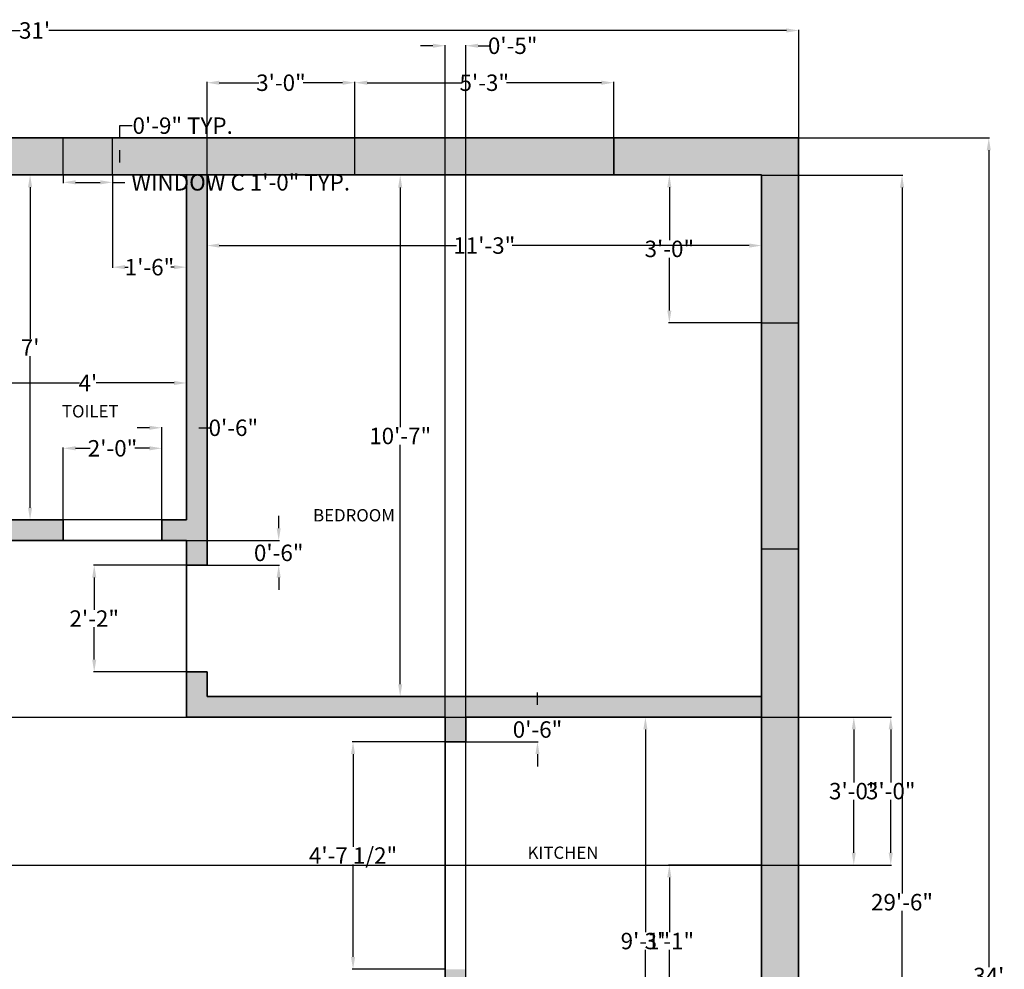
# Model space of a CAD drawing. Units: inches. Extents: x 477 to 929, y 265 to 727.
# Tile 4 of 4: x 690 to 929, y 496 to 727. Entities that reach past the tile are written whole.
import ezdxf

# ---------------------------------------------------------------- set-up
doc = ezdxf.new("R2010")
doc.units = ezdxf.units.IN
doc.header["$MEASUREMENT"] = 0
doc.layers.add('A-ANNO-DIMS', color=215, linetype='Continuous', lineweight=18, true_color=0xa953a0)
doc.layers.add('A-WALL-PATT', color=244, linetype='Continuous', lineweight=13, true_color=0x991b1e)
for name, color, linetype, lineweight in [('A-AREA-IDEN', 3, 'Continuous', 25), ('A-GLAZ', 4, 'Continuous', 25), ('A-GLAZ-PATT', 7, 'Continuous', 13), ('A-WALL', 7, 'Continuous', 35)]:
    doc.layers.add(name, color=color, linetype=linetype, lineweight=lineweight)
doc.styles.get("Standard").update_dxf_attribs({"font": 'arial.ttf'})
doc.dimstyles.get("Standard").update_dxf_attribs({"dimtxt": 4, "dimasz": 3, "dimexe": 0.18, "dimexo": 0.0625, "dimgap": 0.09, "dimtad": 0, "dimtih": 1, "dimtoh": 1, "dimdec": 0, "dimzin": 0, "dimdsep": 46, "dimlunit": 3, "dimtxsty": 'Standard', "dimcen": 0, "dimadec": 0, "dimazin": 0, "dimtfac": 1, "dimtdec": 0, "dimtofl": 0, "dimtmove": 0, "dimatfit": 3, "dimfxl": 1, "dimtolj": 1, "dimtzin": 0, "dimarcsym": 1})

# ---------------------------------------------------------------- blocks, each defined once
blk = doc.blocks.new('*D7')
at = {"layer": 'A-ANNO-DIMS', "color": 0, "lineweight": -2, "transparency": 16777216}
for p, q in [((870.27, 557.21), (841.87, 557.21)), ((842.05, 554.21), (842.05, 504.84)), ((842.05, 451.21), (842.05, 500.57)), ((870.27, 448.21), (841.87, 448.21))]:
    blk.add_line(p, q, dxfattribs=at)
at = {"layer": 'A-ANNO-DIMS', "color": 0, "transparency": 16777216}
for points in [[(841.55, 554.21), (842.55, 554.21), (842.05, 557.21)], [(841.55, 451.21), (842.55, 451.21), (842.05, 448.21)]]:
    blk.add_solid(points, dxfattribs=at)
at = {"layer": 'Defpoints', "color": 0, "transparency": 16777216}
for p in [(870.33, 557.21), (842.05, 448.21), (870.33, 448.21)]:
    blk.add_point(p, dxfattribs=at)
at = {"layer": 'A-ANNO-DIMS', "color": 0, "transparency": 16777216, "insert": (842.05, 502.71), "char_height": 4, "attachment_point": 5}
blk.add_mtext('\\A1;9\'-1"', dxfattribs=at)
blk = doc.blocks.new('*D9')
at = {"layer": 'A-ANNO-DIMS', "color": 0, "lineweight": -2, "transparency": 16777216}
for p, q in [((735.33, 689.14), (735.33, 671.84)), ((870.33, 689.14), (870.33, 671.84)), ((738.33, 672.02), (796.06, 672.02)), ((867.33, 672.02), (809.61, 672.02))]:
    blk.add_line(p, q, dxfattribs=at)
at = {"layer": 'A-ANNO-DIMS', "color": 0, "transparency": 16777216}
for points in [[(738.33, 672.52), (738.33, 671.52), (735.33, 672.02)], [(867.33, 672.52), (867.33, 671.52), (870.33, 672.02)]]:
    blk.add_solid(points, dxfattribs=at)
at = {"layer": 'Defpoints', "color": 0, "transparency": 16777216}
for p in [(735.33, 689.21), (870.33, 689.21), (870.33, 672.02)]:
    blk.add_point(p, dxfattribs=at)
at = {"layer": 'A-ANNO-DIMS', "color": 0, "transparency": 16777216, "insert": (802.83, 672.02), "char_height": 4, "attachment_point": 5}
blk.add_mtext('\\A1;11\'-3"', dxfattribs=at)
blk = doc.blocks.new('*D10')
at = {"layer": 'A-ANNO-DIMS', "color": 0, "lineweight": -2, "transparency": 16777216}
for p, q in [((870.27, 689.14), (782.18, 689.14)), ((782.36, 686.14), (782.36, 627.81)), ((782.36, 565.21), (782.36, 623.54)), ((870.27, 562.21), (782.18, 562.21))]:
    blk.add_line(p, q, dxfattribs=at)
at = {"layer": 'A-ANNO-DIMS', "color": 0, "transparency": 16777216}
for points in [[(781.86, 686.14), (782.86, 686.14), (782.36, 689.14)], [(781.86, 565.21), (782.86, 565.21), (782.36, 562.21)]]:
    blk.add_solid(points, dxfattribs=at)
at = {"layer": 'Defpoints', "color": 0, "transparency": 16777216}
for p in [(870.33, 689.14), (782.36, 562.21), (870.33, 562.21)]:
    blk.add_point(p, dxfattribs=at)
at = {"layer": 'A-ANNO-DIMS', "color": 0, "transparency": 16777216, "insert": (782.36, 625.67), "char_height": 4, "attachment_point": 5}
blk.add_mtext('\\A1;10\'-7"', dxfattribs=at)
blk = doc.blocks.new('*D11')
at = {"layer": 'A-ANNO-DIMS', "color": 0, "lineweight": -2, "transparency": 16777216}
for p, q in [((682.33, 605.27), (682.33, 638.75)), ((685.33, 638.57), (704.32, 638.57)), ((727.33, 638.57), (708.34, 638.57)), ((730.33, 605.27), (730.33, 638.75))]:
    blk.add_line(p, q, dxfattribs=at)
at = {"layer": 'A-ANNO-DIMS', "color": 0, "transparency": 16777216}
for points in [[(685.33, 639.07), (685.33, 638.07), (682.33, 638.57)], [(727.33, 639.07), (727.33, 638.07), (730.33, 638.57)]]:
    blk.add_solid(points, dxfattribs=at)
at = {"layer": 'Defpoints', "color": 0, "transparency": 16777216}
for p in [(730.33, 638.57), (682.33, 605.21), (730.33, 605.21)]:
    blk.add_point(p, dxfattribs=at)
at = {"layer": 'A-ANNO-DIMS', "color": 0, "transparency": 16777216, "insert": (706.33, 638.57), "char_height": 4, "attachment_point": 5}
blk.add_mtext("\\A1;4'", dxfattribs=at)
blk = doc.blocks.new('*D12')
at = {"layer": 'A-ANNO-DIMS', "color": 0, "lineweight": -2, "transparency": 16777216}
for p, q in [((730.27, 689.21), (692.08, 689.21)), ((692.26, 686.21), (692.26, 649.3)), ((692.26, 608.21), (692.26, 645.12)), ((730.27, 605.21), (692.08, 605.21))]:
    blk.add_line(p, q, dxfattribs=at)
at = {"layer": 'A-ANNO-DIMS', "color": 0, "transparency": 16777216}
for points in [[(691.76, 686.21), (692.76, 686.21), (692.26, 689.21)], [(691.76, 608.21), (692.76, 608.21), (692.26, 605.21)]]:
    blk.add_solid(points, dxfattribs=at)
at = {"layer": 'Defpoints', "color": 0, "transparency": 16777216}
for p in [(730.33, 689.21), (692.26, 605.21), (730.33, 605.21)]:
    blk.add_point(p, dxfattribs=at)
at = {"layer": 'A-ANNO-DIMS', "color": 0, "transparency": 16777216, "insert": (692.26, 647.21), "char_height": 4, "attachment_point": 5}
blk.add_mtext("\\A1;7'", dxfattribs=at)
blk = doc.blocks.new('*D17')
at = {"layer": 'A-ANNO-DIMS', "color": 0, "lineweight": -2, "transparency": 16777216}
for p, q in [((879.4, 698.21), (925.82, 698.21)), ((925.64, 695.21), (925.64, 496.34)), ((925.64, 293.21), (925.64, 492.07)), ((879.4, 290.21), (925.82, 290.21))]:
    blk.add_line(p, q, dxfattribs=at)
at = {"layer": 'A-ANNO-DIMS', "color": 0, "transparency": 16777216}
for points in [[(925.14, 695.21), (926.14, 695.21), (925.64, 698.21)], [(925.14, 293.21), (926.14, 293.21), (925.64, 290.21)]]:
    blk.add_solid(points, dxfattribs=at)
at = {"layer": 'Defpoints', "color": 0, "transparency": 16777216}
for p in [(879.33, 698.21), (879.33, 290.21), (925.64, 290.21)]:
    blk.add_point(p, dxfattribs=at)
at = {"layer": 'A-ANNO-DIMS', "color": 0, "transparency": 16777216, "insert": (925.64, 494.21), "char_height": 4, "attachment_point": 5}
blk.add_mtext("\\A1;34'", dxfattribs=at)
blk = doc.blocks.new('*D18')
at = {"layer": 'A-ANNO-DIMS', "color": 0, "lineweight": -2, "transparency": 16777216}
for p, q in [((507.33, 698.27), (507.33, 724.56)), ((510.33, 724.38), (689.88, 724.38)), ((876.4, 724.38), (696.85, 724.38)), ((879.4, 698.27), (879.4, 724.56))]:
    blk.add_line(p, q, dxfattribs=at)
at = {"layer": 'A-ANNO-DIMS', "color": 0, "transparency": 16777216}
for points in [[(510.33, 724.88), (510.33, 723.88), (507.33, 724.38)], [(876.4, 724.88), (876.4, 723.88), (879.4, 724.38)]]:
    blk.add_solid(points, dxfattribs=at)
at = {"layer": 'Defpoints', "color": 0, "transparency": 16777216}
for p in [(879.4, 724.38), (507.33, 698.21), (879.4, 698.21)]:
    blk.add_point(p, dxfattribs=at)
at = {"layer": 'A-ANNO-DIMS', "color": 0, "transparency": 16777216, "insert": (693.36, 724.38), "char_height": 4, "attachment_point": 5}
blk.add_mtext("\\A1;31'", dxfattribs=at)
blk = doc.blocks.new('*D19')
at = {"layer": 'A-ANNO-DIMS', "color": 0, "lineweight": -2, "transparency": 16777216}
for p, q in [((870.4, 689.14), (904.7, 689.14)), ((904.52, 686.14), (904.52, 514.31)), ((904.52, 338.21), (904.52, 510.04)), ((870.33, 335.21), (904.7, 335.21))]:
    blk.add_line(p, q, dxfattribs=at)
at = {"layer": 'A-ANNO-DIMS', "color": 0, "transparency": 16777216}
for points in [[(904.02, 686.14), (905.02, 686.14), (904.52, 689.14)], [(904.02, 338.21), (905.02, 338.21), (904.52, 335.21)]]:
    blk.add_solid(points, dxfattribs=at)
at = {"layer": 'Defpoints', "color": 0, "transparency": 16777216}
for p in [(870.33, 689.14), (870.27, 335.21), (904.52, 335.21)]:
    blk.add_point(p, dxfattribs=at)
at = {"layer": 'A-ANNO-DIMS', "color": 0, "transparency": 16777216, "insert": (904.52, 512.17), "char_height": 4, "attachment_point": 5}
blk.add_mtext('\\A1;29\'-6"', dxfattribs=at)
blk = doc.blocks.new('WIN-JAMBS-55IN')
for p, q in [((0, 55), (9, 55)), ((0, 0), (9, 0))]:
    blk.add_line(p, q)
blk = doc.blocks.new('WIN-JAMBS-12IN')
for p, q in [((0, 0), (0, 9)), ((12, 0), (12, 9))]:
    blk.add_line(p, q)
blk = doc.blocks.new('*D27')
at = {"layer": 'A-ANNO-DIMS', "color": 0, "lineweight": -2, "transparency": 16777216}
for p, q in [((700.33, 689.14), (700.33, 687.23)), ((712.33, 689.14), (712.33, 687.23)), ((703.33, 687.41), (709.33, 687.41)), ((712.33, 687.41), (715.33, 687.41))]:
    blk.add_line(p, q, dxfattribs=at)
at = {"layer": 'A-ANNO-DIMS', "color": 0, "transparency": 16777216}
for points in [[(703.33, 687.91), (703.33, 686.91), (700.33, 687.41)], [(709.33, 687.91), (709.33, 686.91), (712.33, 687.41)]]:
    blk.add_solid(points, dxfattribs=at)
at = {"layer": 'Defpoints', "color": 0, "transparency": 16777216}
for p in [(700.33, 689.21), (712.33, 689.21), (712.33, 687.41)]:
    blk.add_point(p, dxfattribs=at)
at = {"layer": 'A-ANNO-DIMS', "color": 0, "transparency": 16777216, "insert": (743.53, 687.41), "char_height": 4, "attachment_point": 5}
blk.add_mtext('\\A1;WINDOW C 1\'-0" TYP.', dxfattribs=at)
blk = doc.blocks.new('*D28')
at = {"layer": 'A-ANNO-DIMS', "color": 0, "lineweight": -2, "transparency": 16777216}
for p, q in [((714.13, 698.21), (714.13, 701.21)), ((714.13, 701.21), (717.13, 701.21)), ((712.4, 698.21), (714.31, 698.21)), ((714.13, 692.21), (714.13, 695.21)), ((712.4, 689.21), (714.31, 689.21))]:
    blk.add_line(p, q, dxfattribs=at)
at = {"layer": 'A-ANNO-DIMS', "color": 0, "transparency": 16777216}
for points in [[(713.63, 695.21), (714.63, 695.21), (714.13, 698.21)], [(713.63, 692.21), (714.63, 692.21), (714.13, 689.21)]]:
    blk.add_solid(points, dxfattribs=at)
at = {"layer": 'Defpoints', "color": 0, "transparency": 16777216}
for p in [(712.33, 698.21), (714.13, 698.21), (712.33, 689.21)]:
    blk.add_point(p, dxfattribs=at)
at = {"layer": 'A-ANNO-DIMS', "color": 0, "transparency": 16777216, "insert": (729.41, 701.21), "char_height": 4, "attachment_point": 5}
blk.add_mtext('\\A1;0\'-9" TYP.', dxfattribs=at)
blk = doc.blocks.new('*D30')
at = {"layer": 'A-ANNO-DIMS', "color": 0, "lineweight": -2, "transparency": 16777216}
for p, q in [((588.43, 557.21), (901.96, 557.21)), ((901.78, 554.21), (901.78, 541.34)), ((901.78, 524.21), (901.78, 537.07)), ((588.43, 521.21), (901.96, 521.21))]:
    blk.add_line(p, q, dxfattribs=at)
at = {"layer": 'A-ANNO-DIMS', "color": 0, "transparency": 16777216}
for points in [[(901.28, 554.21), (902.28, 554.21), (901.78, 557.21)], [(901.28, 524.21), (902.28, 524.21), (901.78, 521.21)]]:
    blk.add_solid(points, dxfattribs=at)
at = {"layer": 'Defpoints', "color": 0, "transparency": 16777216}
for p in [(588.37, 557.21), (901.78, 557.21), (588.37, 521.21)]:
    blk.add_point(p, dxfattribs=at)
at = {"layer": 'A-ANNO-DIMS', "color": 0, "transparency": 16777216, "insert": (901.78, 539.21), "char_height": 4, "attachment_point": 5}
blk.add_mtext('\\A1;3\'-0"', dxfattribs=at)
blk = doc.blocks.new('*D39')
at = {"layer": 'A-ANNO-DIMS', "color": 0, "lineweight": -2, "transparency": 16777216}
for p, q in [((790.33, 720.66), (787.33, 720.66)), ((793.33, 448.27), (793.33, 720.84)), ((798.33, 448.27), (798.33, 720.84)), ((801.33, 720.66), (804.33, 720.66))]:
    blk.add_line(p, q, dxfattribs=at)
at = {"layer": 'A-ANNO-DIMS', "color": 0, "transparency": 16777216}
for points in [[(790.33, 721.16), (790.33, 720.16), (793.33, 720.66)], [(801.33, 721.16), (801.33, 720.16), (798.33, 720.66)]]:
    blk.add_solid(points, dxfattribs=at)
at = {"layer": 'Defpoints', "color": 0, "transparency": 16777216}
for p in [(798.33, 720.66), (793.33, 448.21), (798.33, 448.21)]:
    blk.add_point(p, dxfattribs=at)
at = {"layer": 'A-ANNO-DIMS', "color": 0, "transparency": 16777216, "insert": (809.74, 720.66), "char_height": 4, "attachment_point": 5}
blk.add_mtext('\\A1;0\'-5"', dxfattribs=at)
blk = doc.blocks.new('*D42')
at = {"layer": 'A-ANNO-DIMS', "color": 0, "lineweight": -2, "transparency": 16777216}
for p, q in [((712.33, 689.14), (712.33, 666.58)), ((730.33, 689.14), (730.33, 666.58)), ((715.33, 666.76), (716.12, 666.76)), ((727.33, 666.76), (726.55, 666.76))]:
    blk.add_line(p, q, dxfattribs=at)
at = {"layer": 'A-ANNO-DIMS', "color": 0, "transparency": 16777216}
for points in [[(715.33, 667.26), (715.33, 666.26), (712.33, 666.76)], [(727.33, 667.26), (727.33, 666.26), (730.33, 666.76)]]:
    blk.add_solid(points, dxfattribs=at)
at = {"layer": 'Defpoints', "color": 0, "transparency": 16777216}
for p in [(712.33, 689.21), (730.33, 689.21), (712.33, 666.76)]:
    blk.add_point(p, dxfattribs=at)
at = {"layer": 'A-ANNO-DIMS', "color": 0, "transparency": 16777216, "insert": (721.33, 666.76), "char_height": 4, "attachment_point": 5}
blk.add_mtext('\\A1;1\'-6"', dxfattribs=at)
blk = doc.blocks.new('*D43')
at = {"layer": 'A-ANNO-DIMS', "color": 0, "lineweight": -2, "transparency": 16777216}
for p, q in [((735.33, 689.27), (735.33, 711.84)), ((738.33, 711.66), (747.93, 711.66)), ((768.33, 711.66), (758.74, 711.66)), ((771.33, 689.27), (771.33, 711.84))]:
    blk.add_line(p, q, dxfattribs=at)
at = {"layer": 'A-ANNO-DIMS', "color": 0, "transparency": 16777216}
for points in [[(738.33, 712.16), (738.33, 711.16), (735.33, 711.66)], [(768.33, 712.16), (768.33, 711.16), (771.33, 711.66)]]:
    blk.add_solid(points, dxfattribs=at)
at = {"layer": 'Defpoints', "color": 0, "transparency": 16777216}
for p in [(771.33, 711.66), (735.33, 689.21), (771.33, 689.21)]:
    blk.add_point(p, dxfattribs=at)
at = {"layer": 'A-ANNO-DIMS', "color": 0, "transparency": 16777216, "insert": (753.33, 711.66), "char_height": 4, "attachment_point": 5}
blk.add_mtext('\\A1;3\'-0"', dxfattribs=at)
blk = doc.blocks.new('*D44')
at = {"layer": 'A-ANNO-DIMS', "color": 0, "lineweight": -2, "transparency": 16777216}
for p, q in [((771.33, 689.27), (771.33, 711.84)), ((774.33, 711.66), (797.43, 711.66)), ((831.33, 711.66), (808.24, 711.66)), ((834.33, 689.27), (834.33, 711.84))]:
    blk.add_line(p, q, dxfattribs=at)
at = {"layer": 'A-ANNO-DIMS', "color": 0, "transparency": 16777216}
for points in [[(774.33, 712.16), (774.33, 711.16), (771.33, 711.66)], [(831.33, 712.16), (831.33, 711.16), (834.33, 711.66)]]:
    blk.add_solid(points, dxfattribs=at)
at = {"layer": 'Defpoints', "color": 0, "transparency": 16777216}
for p in [(834.33, 711.66), (771.33, 689.21), (834.33, 689.21)]:
    blk.add_point(p, dxfattribs=at)
at = {"layer": 'A-ANNO-DIMS', "color": 0, "transparency": 16777216, "insert": (802.83, 711.66), "char_height": 4, "attachment_point": 5}
blk.add_mtext('\\A1;5\'-3"', dxfattribs=at)
blk = doc.blocks.new('*D50')
at = {"layer": 'A-ANNO-DIMS', "color": 0, "lineweight": -2, "transparency": 16777216}
for p, q in [((870.27, 689.21), (847.7, 689.21)), ((847.88, 686.21), (847.88, 673.34)), ((847.88, 656.21), (847.88, 669.07)), ((870.27, 653.21), (847.7, 653.21))]:
    blk.add_line(p, q, dxfattribs=at)
at = {"layer": 'A-ANNO-DIMS', "color": 0, "transparency": 16777216}
for points in [[(847.38, 686.21), (848.38, 686.21), (847.88, 689.21)], [(847.38, 656.21), (848.38, 656.21), (847.88, 653.21)]]:
    blk.add_solid(points, dxfattribs=at)
at = {"layer": 'Defpoints', "color": 0, "transparency": 16777216}
for p in [(847.88, 689.21), (870.33, 689.21), (870.33, 653.21)]:
    blk.add_point(p, dxfattribs=at)
at = {"layer": 'A-ANNO-DIMS', "color": 0, "transparency": 16777216, "insert": (847.88, 671.21), "char_height": 4, "attachment_point": 5}
blk.add_mtext('\\A1;3\'-0"', dxfattribs=at)
blk = doc.blocks.new('*D51')
at = {"layer": 'A-ANNO-DIMS', "color": 0, "lineweight": -2, "transparency": 16777216}
for p, q in [((870.4, 557.21), (892.96, 557.21)), ((892.78, 554.21), (892.78, 541.34)), ((892.78, 524.21), (892.78, 537.07)), ((870.4, 521.21), (892.96, 521.21))]:
    blk.add_line(p, q, dxfattribs=at)
at = {"layer": 'A-ANNO-DIMS', "color": 0, "transparency": 16777216}
for points in [[(892.28, 554.21), (893.28, 554.21), (892.78, 557.21)], [(892.28, 524.21), (893.28, 524.21), (892.78, 521.21)]]:
    blk.add_solid(points, dxfattribs=at)
at = {"layer": 'Defpoints', "color": 0, "transparency": 16777216}
for p in [(870.33, 557.21), (870.33, 521.21), (892.78, 521.21)]:
    blk.add_point(p, dxfattribs=at)
at = {"layer": 'A-ANNO-DIMS', "color": 0, "transparency": 16777216, "insert": (892.78, 539.21), "char_height": 4, "attachment_point": 5}
blk.add_mtext('\\A1;3\'-0"', dxfattribs=at)
blk = doc.blocks.new('*D52')
at = {"layer": 'A-ANNO-DIMS', "color": 0, "lineweight": -2, "transparency": 16777216}
for p, q in [((870.27, 521.21), (847.7, 521.21)), ((847.88, 518.21), (847.88, 504.84)), ((847.88, 487.21), (847.88, 500.57)), ((870.27, 484.21), (847.7, 484.21))]:
    blk.add_line(p, q, dxfattribs=at)
at = {"layer": 'A-ANNO-DIMS', "color": 0, "transparency": 16777216}
for points in [[(847.38, 518.21), (848.38, 518.21), (847.88, 521.21)], [(847.38, 487.21), (848.38, 487.21), (847.88, 484.21)]]:
    blk.add_solid(points, dxfattribs=at)
at = {"layer": 'Defpoints', "color": 0, "transparency": 16777216}
for p in [(847.88, 521.21), (870.33, 521.21), (870.33, 484.21)]:
    blk.add_point(p, dxfattribs=at)
at = {"layer": 'A-ANNO-DIMS', "color": 0, "transparency": 16777216, "insert": (847.88, 502.71), "char_height": 4, "attachment_point": 5}
blk.add_mtext('\\A1;3\'-1"', dxfattribs=at)
blk = doc.blocks.new('*D59')
at = {"layer": 'A-ANNO-DIMS', "color": 0, "lineweight": -2, "transparency": 16777216}
for p, q in [((793.27, 551.21), (770.7, 551.21)), ((770.88, 548.21), (770.88, 525.68)), ((770.88, 498.83), (770.88, 521.36)), ((793.27, 495.83), (770.7, 495.83))]:
    blk.add_line(p, q, dxfattribs=at)
at = {"layer": 'A-ANNO-DIMS', "color": 0, "transparency": 16777216}
for points in [[(770.38, 548.21), (771.38, 548.21), (770.88, 551.21)], [(770.38, 498.83), (771.38, 498.83), (770.88, 495.83)]]:
    blk.add_solid(points, dxfattribs=at)
at = {"layer": 'Defpoints', "color": 0, "transparency": 16777216}
for p in [(770.88, 551.21), (793.33, 551.21), (793.33, 495.83)]:
    blk.add_point(p, dxfattribs=at)
at = {"layer": 'A-ANNO-DIMS', "color": 0, "transparency": 16777216, "insert": (770.88, 523.52), "char_height": 4, "attachment_point": 5}
blk.add_mtext('\\A1;4\'-7 1/2"', dxfattribs=at)
blk = doc.blocks.new('*D60')
at = {"layer": 'A-ANNO-DIMS', "color": 0, "lineweight": -2, "transparency": 16777216}
for p, q in [((730.27, 594.21), (707.7, 594.21)), ((707.88, 591.21), (707.88, 583.3)), ((707.88, 571.21), (707.88, 579.11)), ((730.27, 568.21), (707.7, 568.21))]:
    blk.add_line(p, q, dxfattribs=at)
at = {"layer": 'A-ANNO-DIMS', "color": 0, "transparency": 16777216}
for points in [[(707.38, 591.21), (708.38, 591.21), (707.88, 594.21)], [(707.38, 571.21), (708.38, 571.21), (707.88, 568.21)]]:
    blk.add_solid(points, dxfattribs=at)
at = {"layer": 'Defpoints', "color": 0, "transparency": 16777216}
for p in [(707.88, 594.21), (730.33, 594.21), (730.33, 568.21)]:
    blk.add_point(p, dxfattribs=at)
at = {"layer": 'A-ANNO-DIMS', "color": 0, "transparency": 16777216, "insert": (707.88, 581.21), "char_height": 4, "attachment_point": 5}
blk.add_mtext('\\A1;2\'-2"', dxfattribs=at)
blk = doc.blocks.new('*D62')
at = {"layer": 'A-ANNO-DIMS', "color": 0, "lineweight": -2, "transparency": 16777216}
for p, q in [((700.33, 600.27), (700.33, 622.84)), ((703.33, 622.66), (706.89, 622.66)), ((721.33, 622.66), (717.77, 622.66)), ((724.33, 600.27), (724.33, 622.84))]:
    blk.add_line(p, q, dxfattribs=at)
at = {"layer": 'A-ANNO-DIMS', "color": 0, "transparency": 16777216}
for points in [[(703.33, 623.16), (703.33, 622.16), (700.33, 622.66)], [(721.33, 623.16), (721.33, 622.16), (724.33, 622.66)]]:
    blk.add_solid(points, dxfattribs=at)
at = {"layer": 'Defpoints', "color": 0, "transparency": 16777216}
for p in [(724.33, 622.66), (700.33, 600.21), (724.33, 600.21)]:
    blk.add_point(p, dxfattribs=at)
at = {"layer": 'A-ANNO-DIMS', "color": 0, "transparency": 16777216, "insert": (712.33, 622.66), "char_height": 4, "attachment_point": 5}
blk.add_mtext('\\A1;2\'-0"', dxfattribs=at)
blk = doc.blocks.new('*D66')
at = {"layer": 'A-ANNO-DIMS', "color": 0, "lineweight": -2, "transparency": 16777216}
for p, q in [((752.783739, 603.205163), (752.783739, 606.205163)), ((730.396239, 600.205163), (752.963739, 600.205163)), ((730.396239, 594.205163), (752.963739, 594.205163)), ((752.783739, 591.205163), (752.783739, 588.205163))]:
    blk.add_line(p, q, dxfattribs=at)
at = {"layer": 'A-ANNO-DIMS', "color": 0, "transparency": 16777216}
for points in [[(752.283739, 603.205163), (753.283739, 603.205163), (752.783739, 600.205163)], [(752.283739, 591.205163), (753.283739, 591.205163), (752.783739, 594.205163)]]:
    blk.add_solid(points, dxfattribs=at)
at = {"layer": 'Defpoints', "color": 0, "transparency": 16777216}
for p in [(730.333739, 600.205163), (730.333739, 594.205163), (752.783739, 594.205163)]:
    blk.add_point(p, dxfattribs=at)
at = {"layer": 'A-ANNO-DIMS', "color": 0, "transparency": 16777216, "insert": (752.783739, 597.205163), "char_height": 4, "attachment_point": 5}
blk.add_mtext('\\A1;0\'-6"', dxfattribs=at)
blk = doc.blocks.new('*D69')
at = {"layer": 'A-ANNO-DIMS', "color": 0, "lineweight": -2, "transparency": 16777216}
for p, q in [((721.33, 627.66), (718.33, 627.66)), ((724.33, 605.27), (724.33, 627.84)), ((730.33, 605.27), (730.33, 627.84)), ((733.33, 627.66), (736.33, 627.66))]:
    blk.add_line(p, q, dxfattribs=at)
at = {"layer": 'A-ANNO-DIMS', "color": 0, "transparency": 16777216}
for points in [[(721.33, 628.16), (721.33, 627.16), (724.33, 627.66)], [(733.33, 628.16), (733.33, 627.16), (730.33, 627.66)]]:
    blk.add_solid(points, dxfattribs=at)
at = {"layer": 'Defpoints', "color": 0, "transparency": 16777216}
for p in [(730.33, 627.66), (724.33, 605.21), (730.33, 605.21)]:
    blk.add_point(p, dxfattribs=at)
at = {"layer": 'A-ANNO-DIMS', "color": 0, "transparency": 16777216, "insert": (741.74, 627.66), "char_height": 4, "attachment_point": 5}
blk.add_mtext('\\A1;0\'-6"', dxfattribs=at)
blk = doc.blocks.new('*D70')
at = {"layer": 'A-ANNO-DIMS', "color": 0, "lineweight": -2, "transparency": 16777216}
for p, q in [((815.783739, 560.205163), (815.783739, 563.205163)), ((793.396239, 557.205163), (815.963739, 557.205163)), ((793.396239, 551.205163), (815.963739, 551.205163)), ((815.783739, 548.205163), (815.783739, 545.205163))]:
    blk.add_line(p, q, dxfattribs=at)
at = {"layer": 'A-ANNO-DIMS', "color": 0, "transparency": 16777216}
for points in [[(815.283739, 560.205163), (816.283739, 560.205163), (815.783739, 557.205163)], [(815.283739, 548.205163), (816.283739, 548.205163), (815.783739, 551.205163)]]:
    blk.add_solid(points, dxfattribs=at)
at = {"layer": 'Defpoints', "color": 0, "transparency": 16777216}
for p in [(793.333739, 557.205163), (793.333739, 551.205163), (815.783739, 551.205163)]:
    blk.add_point(p, dxfattribs=at)
at = {"layer": 'A-ANNO-DIMS', "color": 0, "transparency": 16777216, "insert": (815.783739, 554.205163), "char_height": 4, "attachment_point": 5}
blk.add_mtext('\\A1;0\'-6"', dxfattribs=at)

msp = doc.modelspace()

# ---------------------------------------------------------------- hatches: boundary and pattern name
at = {"layer": 'A-GLAZ-PATT'}
h = msp.add_hatch(color=256, dxfattribs=at)
h.dxf.hatch_style = 1
h.paths.add_polyline_path([(588.33, 698.21), (552.33, 698.21), (552.33, 689.21), (588.33, 689.21)])
h.paths.add_polyline_path([(659.33, 698.21), (647.33, 698.21), (647.33, 689.21), (659.33, 689.21)])
h.paths.add_polyline_path([(712.33, 698.21), (700.33, 698.21), (700.33, 689.21), (712.33, 689.21)])
h.paths.add_polyline_path([(834.33, 698.21), (771.33, 698.21), (771.33, 689.21), (834.33, 689.21)])
h.paths.add_polyline_path([(879.33, 653.21), (870.33, 653.21), (870.33, 598.21), (879.33, 598.21)])
h.paths.add_polyline_path([(879.33, 521.21), (870.33, 521.21), (870.33, 484.21), (879.33, 484.21)])
h.paths.add_polyline_path([(879.33, 407.21), (870.33, 407.21), (870.33, 371.21), (879.33, 371.21)])
h.paths.add_polyline_path([(834.33, 335.21), (766.33, 335.21), (766.33, 326.21), (834.33, 326.21)])
h.paths.add_polyline_path([(588.33, 335.21), (552.33, 335.21), (552.33, 326.21), (588.33, 326.21)])
h.paths.add_polyline_path([(516.33, 430.21), (507.33, 430.21), (507.33, 371.21), (516.33, 371.21)])
h.paths.add_polyline_path([(516.33, 539.21), (507.33, 539.21), (507.33, 466.21), (516.33, 466.21)])
h.paths.add_polyline_path([(516.33, 653.21), (507.33, 653.21), (507.33, 598.21), (516.33, 598.21)])
at = {"layer": 'A-WALL-PATT'}
h = msp.add_hatch(color=256, dxfattribs=at)
h.dxf.hatch_style = 1
h.paths.add_polyline_path([(516.33, 598.21), (507.33, 598.21), (507.33, 539.21), (516.33, 539.21), (516.33, 557.21), (570.33, 557.21), (570.33, 562.21), (516.33, 562.21)])
h.paths.add_polyline_path([(552.33, 698.21), (507.33, 698.21), (507.33, 653.21), (516.33, 653.21), (516.33, 689.21), (552.33, 689.21)])
h.paths.add_polyline_path([(647.33, 698.21), (588.33, 698.21), (588.33, 689.21), (647.33, 689.21)])
h.paths.add_polyline_path([(700.33, 698.21), (659.33, 698.21), (659.33, 689.21), (700.33, 689.21)])
h.paths.add_polyline_path([(771.33, 698.21), (712.33, 698.21), (712.33, 689.21), (771.33, 689.21)])
h.paths.add_polyline_path([(879.33, 698.21), (834.33, 698.21), (834.33, 689.21), (870.33, 689.21), (870.33, 653.21), (879.33, 653.21)])
h.paths.add_polyline_path([(879.33, 598.21), (870.33, 598.21), (870.33, 562.21), (735.33, 562.21), (735.33, 568.21), (730.33, 568.21), (730.33, 557.21), (793.33, 557.21), (793.33, 551.21), (798.33, 551.21), (798.33, 557.21), (870.33, 557.21), (870.33, 521.21), (879.33, 521.21)])
h.paths.add_polyline_path([(879.33, 484.21), (870.33, 484.21), (870.33, 448.21), (798.33, 448.21), (798.33, 495.83), (793.33, 495.83), (793.33, 448.21), (788.33, 448.21), (788.33, 443.21), (870.33, 443.21), (870.33, 407.21), (879.33, 407.21)])
h.paths.add_polyline_path([(735.33, 443.21), (740.33, 443.21), (740.33, 448.21), (730.33, 448.21), (730.33, 400.21), (682.33, 400.21), (682.33, 395.21), (730.33, 395.21), (730.33, 326.21), (766.33, 326.21), (766.33, 335.21), (735.33, 335.21)])
h.paths.add_polyline_path([(879.33, 371.21), (870.33, 371.21), (870.33, 335.21), (834.33, 335.21), (834.33, 326.21), (879.33, 326.21)])
h.paths.add_polyline_path([(516.33, 466.21), (507.33, 466.21), (507.33, 430.21), (516.33, 430.21), (516.33, 443.21), (624.33, 443.21), (624.33, 437.21), (629.33, 437.21), (629.33, 448.21), (516.33, 448.21)])
h.paths.add_polyline_path([(629.33, 600.21), (700.33, 600.21), (700.33, 605.21), (682.33, 605.21), (682.33, 689.21), (677.33, 689.21), (677.33, 605.21), (629.33, 605.21), (629.33, 611.21), (624.33, 611.21), (624.33, 562.21), (618.33, 562.21), (618.33, 557.21), (629.33, 557.21)])
h.paths.add_polyline_path([(629.33, 689.21), (624.33, 689.21), (624.33, 653.21), (629.33, 653.21)], flags=17)
h = msp.add_hatch(color=256, dxfattribs=at)
h.dxf.hatch_style = 1
h.paths.add_polyline_path([(735.33, 689.21), (730.33, 689.21), (730.33, 605.21), (724.33, 605.21), (724.33, 600.21), (730.33, 600.21), (730.33, 594.21), (735.33, 594.21)])

# ---------------------------------------------------------------- linework, layer by layer
at = {"layer": 'A-GLAZ'}
for p, q in [((771.33, 689.21), (771.33, 698.21)), ((834.33, 698.21), (834.33, 689.21)), ((870.33, 521.21), (879.33, 521.21))]:
    msp.add_line(p, q, dxfattribs=at)
at = {"layer": 'A-WALL'}
for p, q in [((507.33, 698.21), (879.33, 698.21)), ((879.33, 698.21), (507.33, 698.21)), ((879.33, 698.21), (879.33, 326.21)), ((879.33, 698.21), (879.33, 326.21)), ((516.33, 689.21), (870.33, 689.21)), ((516.33, 689.21), (870.33, 689.21)), ((730.33, 605.21), (730.33, 689.21)), ((735.33, 594.21), (735.33, 689.21)), ((870.33, 689.21), (870.33, 448.21)), ((682.33, 605.21), (700.33, 605.21)), ((700.33, 600.21), (700.33, 605.21)), ((724.33, 600.21), (724.33, 605.21)), ((724.33, 605.21), (730.33, 605.21)), ((629.33, 600.21), (730.33, 600.21)), ((730.33, 557.21), (730.33, 600.21)), ((730.33, 594.21), (735.33, 594.21)), ((730.33, 568.21), (735.33, 568.21)), ((735.33, 562.21), (735.33, 568.21)), ((735.33, 562.21), (870.33, 562.21)), ((782.18, 562.21), (870.33, 562.21)), ((730.33, 557.21), (793.33, 557.21)), ((793.33, 557.21), (793.33, 448.21)), ((798.33, 557.21), (798.33, 551.21)), ((798.33, 557.21), (870.33, 557.21)), ((841.87, 557.21), (870.27, 557.21)), ((870.33, 557.21), (870.33, 448.21)), ((793.33, 551.21), (798.33, 551.21))]:
    msp.add_line(p, q, dxfattribs=at)

# ---------------------------------------------------------------- block references
at = {"layer": 'A-GLAZ'}
for name, p in [('WIN-JAMBS-12IN', (700.33, 689.21)), ('WIN-JAMBS-55IN', (870.33, 598.21))]:
    msp.add_blockref(name, p, dxfattribs=at)

# ---------------------------------------------------------------- texts
at = {"layer": 'A-AREA-IDEN'}
for s, p in [('TOILET', (700.02, 630.17)), ('KITCHEN', (813.37, 522.72))]:
    msp.add_text(s, height=3, dxfattribs=at).set_placement(p)
at = {"layer": 'A-AREA-IDEN', "insert": (761.16, 607.86), "char_height": 3, "attachment_point": 1}
msp.add_mtext_dynamic_manual_height_columns('BEDROOM', width=102.2555, gutter_width=1, heights=[0], dxfattribs=at)

# ---------------------------------------------------------------- dimensions: what is measured, and where the dimension line sits
at = {"layer": 'A-ANNO-DIMS'}
for base, p1, p2, override, picture, middle in [((879.4, 724.38), (507.33, 698.21), (879.4, 698.21), {"dimclrd": 0, "dimclre": 0, "dimclrt": 0}, '*D18', (693.36, 724.38)), ((798.33, 720.66), (793.33, 448.21), (798.33, 448.21), {"dimdec": 1, "dimlfac": 1, "dimrnd": 0, "dimzin": 1, "dimdsep": 46, "dimlunit": 4, "dimfrac": 2}, '*D39', (809.74, 720.66)), ((834.33, 711.66), (771.33, 689.21), (834.33, 689.21), {"dimdec": 1, "dimlfac": 1, "dimrnd": 0, "dimzin": 1, "dimdsep": 46, "dimlunit": 4, "dimfrac": 2}, '*D44', (802.83, 711.66)), ((870.33, 672.02), (735.33, 689.21), (870.33, 689.21), {"dimclrd": 0, "dimclre": 0, "dimclrt": 0}, '*D9', (802.83, 672.02)), ((730.33, 638.57), (682.33, 605.21), (730.33, 605.21), {"dimclrd": 0, "dimclre": 0, "dimclrt": 0}, '*D11', (706.33, 638.57)), ((730.33, 627.66), (724.33, 605.21), (730.33, 605.21), {"dimdec": 1, "dimlfac": 1, "dimrnd": 0, "dimzin": 1, "dimdsep": 46, "dimlunit": 4, "dimfrac": 2}, '*D69', (741.74, 627.66)), ((724.33, 622.66), (700.33, 600.21), (724.33, 600.21), {"dimdec": 1, "dimlfac": 1, "dimrnd": 0, "dimzin": 1, "dimdsep": 46, "dimlunit": 4, "dimfrac": 2}, '*D62', (712.33, 622.66))]:
    dim = msp.add_linear_dim(base=base, p1=p1, p2=p2, dimstyle='Standard', override=override, dxfattribs=at)
    dim.commit()
    dim.dimension.update_dxf_attribs({"geometry": picture, "text_midpoint": middle})
for base, p1, p2, angle, override, picture, middle in [((771.33, 711.66), (735.33, 689.21), (771.33, 689.21), 0, {"dimdec": 1, "dimlfac": 1, "dimrnd": 0, "dimzin": 1, "dimdsep": 46, "dimlunit": 4, "dimfrac": 2}, '*D43', (753.33, 711.66)), ((925.64, 290.21), (879.33, 698.21), (879.33, 290.21), 90, {"dimclrd": 0, "dimclre": 0, "dimclrt": 0}, '*D17', (925.64, 494.21)), ((692.26, 605.21), (730.33, 689.21), (730.33, 605.21), 90, {"dimclrd": 0, "dimclre": 0, "dimclrt": 0}, '*D12', (692.26, 647.21)), ((712.33, 666.76), (730.33, 689.21), (712.33, 689.21), 180, {"dimdec": 1, "dimlfac": 1, "dimrnd": 0, "dimzin": 1, "dimdsep": 46, "dimlunit": 4, "dimfrac": 2}, '*D42', (721.33, 666.76)), ((782.36, 562.21), (870.33, 689.14), (870.33, 562.21), 90, {"dimclrd": 0, "dimclre": 0, "dimclrt": 0}, '*D10', (782.36, 625.67)), ((847.88, 689.21), (870.33, 653.21), (870.33, 689.21), 90, {"dimdec": 1, "dimlfac": 1, "dimrnd": 0, "dimzin": 1, "dimdsep": 46, "dimlunit": 4, "dimfrac": 2}, '*D50', (847.88, 671.21)), ((904.52, 335.21), (870.33, 689.14), (870.27, 335.21), 90, {"dimclrd": 0, "dimclre": 0, "dimclrt": 0}, '*D19', (904.52, 512.17)), ((752.78, 594.21), (730.33, 600.21), (730.33, 594.21), 270, {"dimdec": 1, "dimlfac": 1, "dimrnd": 0, "dimzin": 1, "dimdsep": 46, "dimlunit": 4, "dimfrac": 2}, '*D66', (752.78, 597.21)), ((707.88, 594.21), (730.33, 568.21), (730.33, 594.21), 90, {"dimdec": 1, "dimlfac": 1, "dimrnd": 0, "dimzin": 1, "dimdsep": 46, "dimlunit": 4, "dimfrac": 2}, '*D60', (707.88, 581.21)), ((815.78, 551.21), (793.33, 557.21), (793.33, 551.21), 270, {"dimdec": 1, "dimlfac": 1, "dimrnd": 0, "dimzin": 1, "dimdsep": 46, "dimlunit": 4, "dimfrac": 2}, '*D70', (815.78, 554.21)), ((901.78, 557.21), (588.37, 521.21), (588.37, 557.21), 90, {"dimdec": 1, "dimlfac": 1, "dimrnd": 0, "dimzin": 1, "dimdsep": 46, "dimlunit": 4, "dimfrac": 2}, '*D30', (901.78, 539.21)), ((842.05, 448.21), (870.33, 557.21), (870.33, 448.21), 90, {"dimclrd": 0, "dimclre": 0, "dimclrt": 0}, '*D7', (842.05, 502.71)), ((892.78, 521.21), (870.33, 557.21), (870.33, 521.21), 270, {"dimdec": 1, "dimlfac": 1, "dimrnd": 0, "dimzin": 1, "dimdsep": 46, "dimlunit": 4, "dimfrac": 2}, '*D51', (892.78, 539.21)), ((770.88, 551.21), (793.33, 495.83), (793.33, 551.21), 90, {"dimdec": 1, "dimlfac": 1, "dimrnd": 0, "dimzin": 1, "dimdsep": 46, "dimlunit": 4, "dimfrac": 2}, '*D59', (770.88, 523.52)), ((847.88, 521.21), (870.33, 484.21), (870.33, 521.21), 90, {"dimdec": 1, "dimlfac": 1, "dimrnd": 0, "dimzin": 1, "dimdsep": 46, "dimlunit": 4, "dimfrac": 2}, '*D52', (847.88, 502.71))]:
    dim = msp.add_linear_dim(base=base, p1=p1, p2=p2, angle=angle, dimstyle='Standard', override=override, dxfattribs=at)
    dim.commit()
    dim.dimension.update_dxf_attribs({"geometry": picture, "text_midpoint": middle})
dim = msp.add_linear_dim(base=(714.13, 698.21), p1=(712.33, 689.21), p2=(712.33, 698.21), angle=90, text='<> TYP.', dimstyle='Standard', override={"dimdec": 1, "dimlfac": 1, "dimrnd": 0, "dimzin": 1, "dimdsep": 46, "dimlunit": 4, "dimfrac": 2}, dxfattribs=at)
dim.commit()
dim.dimension.update_dxf_attribs({"geometry": '*D28', "text_midpoint": (729.41, 701.21)})
dim = msp.add_linear_dim(base=(712.33, 687.41), p1=(700.33, 689.21), p2=(712.33, 689.21), text='WINDOW C <> TYP.', dimstyle='Standard', override={"dimdec": 1, "dimlfac": 1, "dimrnd": 0, "dimzin": 1, "dimdsep": 46, "dimlunit": 4, "dimfrac": 2}, dxfattribs=at)
dim.commit()
dim.dimension.update_dxf_attribs({"geometry": '*D27', "text_midpoint": (743.53, 687.41)})

doc.saveas('drawing.dxf')
